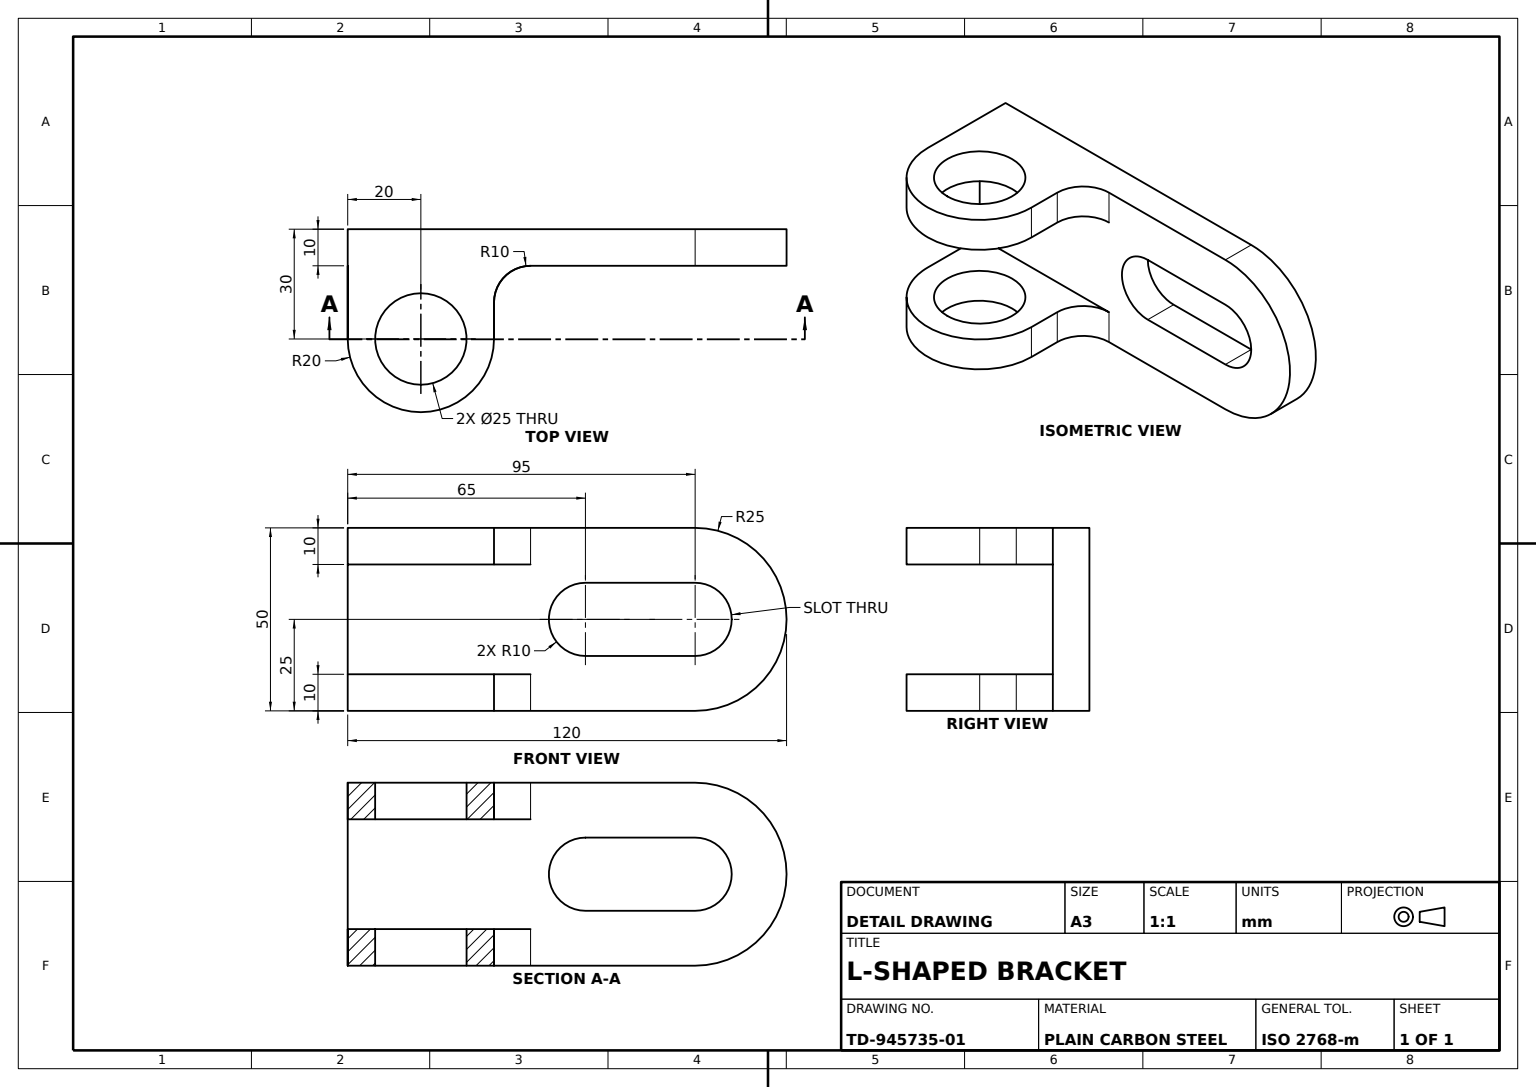
SolidWorks part; units mm, degrees
material "Plain Carbon Steel"
ref_plane "Front Plane" through (0, 0, 0) normal (0, 0, 1) x (1, 0, 0)
ref_plane "Top Plane" through (0, 0, 0) normal (0, 1, 0) x (1, 0, 0)
ref_plane "Right Plane" through (0, 0, 0) normal (1, 0, 0) x (0, 0, -1)
sketch "Base Plate Sketch" plane through (0, 0, 0) normal (0, 0, 1) x (1, 0, 0)
  line L2 (95, 25) -> (0, 25)
  line L3 (0, 25) -> (0, -25)
  line L4 (0, -25) -> (95, -25)
  arc A0 (95, -25) -> (95, 25) centre (95, 0) ccw
  dimension "D1" = 50
  dimension "D2" = 95
  dimension "D3" = 25
  dimension "D4" = 50
extrude "Base Plate" add sketch "Base Plate Sketch" along normal blind 10
sketch "Slot Sketch" plane through (0, 0, 10) normal (0, 0, 1) x (1, 0, 0)
  line L1 (65, 10) -> (95, 10)
  line L3 (95, -10) -> (65, -10)
  arc A0 (65, 10) -> (65, -10) centre (65, 0) ccw
  arc A1 (95, -10) -> (95, 10) centre (95, 0) ccw
  dimension "D1" = 20
  dimension "D2" = 20
  dimension "D3" = 10
  dimension "D4" = 65
extrude "Slot Cut" cut sketch "Slot Sketch" against normal blind 10
sketch "Lug 1 Sketch" plane through (0, -25, 0) normal (0, -1, 0) x (1, 0, 0)
  line L0 (0, 10) -> (0, 30)
  line L1 (0, 10) -> (50, 10)
  line L2 (40, 30) -> (40, 20)
  line L3 (0, 10) -> (95, 10) construction
  arc A0 (40, 30) -> (0, 30) centre (20, 30) ccw
  arc A1 (50, 10) -> (40, 20) centre (50, 20) cw
  point P12 (40, 10)
  dimension "D1" = 40
  dimension "D2" = 10
extrude "Lug 1" add sketch "Lug 1 Sketch" against normal blind 10
sketch "Lug 2 Sketch" plane through (0, 25, 0) normal (0, 1, 0) x (1, 0, 0)
  line L0 (0, -30) -> (0, -10)
  line L1 (0, -10) -> (0, 0) construction
  line L2 (40, -30) -> (40, -20)
  line L3 (0, -10) -> (50, -10)
  line L4 (95, 0) -> (0, 0) construction
  arc A0 (0, -30) -> (40, -30) centre (20, -30) ccw
  arc A1 (50, -10) -> (40, -20) centre (50, -20) ccw
  dimension "D1" = 40
  dimension "D2" = 10
  dimension "D3" = 20
  dimension "D4" = 20
  dimension "D5" = 10
extrude "Lug 2" add sketch "Lug 2 Sketch" against normal blind 10
sketch "Pin Hole Sketch" plane through (0, -25, 0) normal (0, -1, 0) x (1, 0, 0)
  circle A0 centre (20, 30) radius 12.5
  dimension "D1" = 25
  dimension "D2" = 25
extrude "Pin Hole Ø25" cut sketch "Pin Hole Sketch" against normal blind 50
